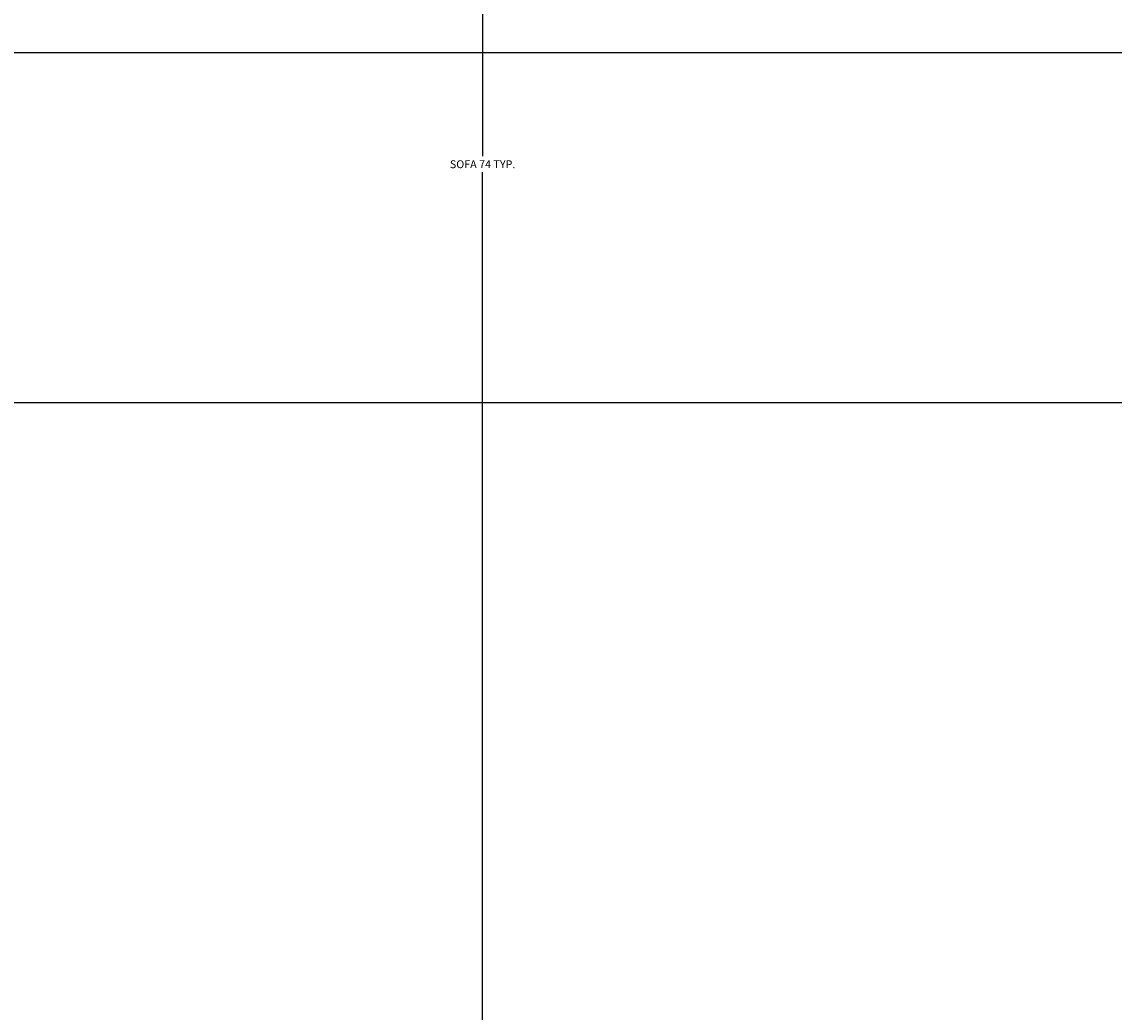
# Model space of a CAD drawing. Units: inches. Extents: x 1998 to 2588, y 1139 to 1977.
# Tile 46 of 134: x 2257 to 2282, y 1615 to 1637. Entities that reach past the tile are written whole.
import ezdxf

# ---------------------------------------------------------------- set-up
doc = ezdxf.new("R2010")
doc.units = ezdxf.units.IN
doc.layers.add('A-ANNO-DIMS', color=2, linetype='Continuous', lineweight=18)
doc.styles.get("Standard").update_dxf_attribs({"font": 'arial.ttf'})
doc.dimstyles.get("Standard").update_dxf_attribs({"dimtxt": 0.18, "dimasz": 0.18, "dimexe": 0.18, "dimexo": 0.0625, "dimgap": 0.09, "dimtad": 0, "dimtih": 1, "dimtoh": 1, "dimdec": 4, "dimzin": 0, "dimdsep": 46, "dimtxsty": 'Standard', "dimcen": 0.09, "dimadec": 0, "dimazin": 0, "dimtfac": 1, "dimtdec": 4, "dimtofl": 0, "dimtmove": 0, "dimatfit": 3, "dimfxl": 1, "dimtolj": 1, "dimtzin": 0, "dimarcsym": 0})

# ---------------------------------------------------------------- blocks, each defined once
blk = doc.blocks.new('*D11')
at = {"layer": 'A-ANNO-DIMS', "color": 0, "lineweight": -2, "transparency": 16777216}
for p, q in [((2256.378, 1671.356), (2267.646, 1671.356)), ((2267.466, 1671.176), (2267.466, 1634.372)), ((2267.466, 1597.201), (2267.466, 1634.005)), ((2256.378, 1597.021), (2267.646, 1597.021))]:
    blk.add_line(p, q, dxfattribs=at)
at = {"layer": 'A-ANNO-DIMS', "color": 0, "transparency": 16777216}
for points in [[(2267.436, 1671.176), (2267.496, 1671.176), (2267.466, 1671.356)], [(2267.436, 1597.201), (2267.496, 1597.201), (2267.466, 1597.021)]]:
    blk.add_solid(points, dxfattribs=at)
at = {"layer": 'Defpoints', "color": 0, "transparency": 16777216}
for p in [(2256.316, 1671.356), (2256.316, 1597.021), (2267.466, 1597.021)]:
    blk.add_point(p, dxfattribs=at)
at = {"layer": 'A-ANNO-DIMS', "color": 0, "transparency": 16777216, "insert": (2267.466, 1634.189), "char_height": 0.18, "attachment_point": 5}
blk.add_mtext('\\A1;SOFA 74 TYP.', dxfattribs=at)
blk = doc.blocks.new('*D30')
at = {"layer": 'A-ANNO-DIMS', "color": 0, "lineweight": -2, "transparency": 16777216}
for p, q in [((2407.91, 1636.732), (1997.843, 1636.732)), ((1998.023, 1636.552), (1998.023, 1615.913)), ((1998.023, 1594.912), (1998.023, 1615.552)), ((2407.91, 1594.732), (1997.843, 1594.732))]:
    blk.add_line(p, q, dxfattribs=at)
at = {"layer": 'A-ANNO-DIMS', "color": 0, "transparency": 16777216}
for points in [[(1997.993, 1636.552), (1998.053, 1636.552), (1998.023, 1636.732)], [(1997.993, 1594.912), (1998.053, 1594.912), (1998.023, 1594.732)]]:
    blk.add_solid(points, dxfattribs=at)
at = {"layer": 'Defpoints', "color": 0, "transparency": 16777216}
for p in [(1998.023, 1636.732), (2407.973, 1636.732), (2407.973, 1594.732)]:
    blk.add_point(p, dxfattribs=at)
at = {"layer": 'A-ANNO-DIMS', "color": 0, "transparency": 16777216, "insert": (1998.023, 1615.732), "char_height": 0.18, "attachment_point": 5}
blk.add_mtext('\\A1;42', dxfattribs=at)
blk = doc.blocks.new('*D39')
at = {"layer": 'A-ANNO-DIMS', "color": 0, "lineweight": -2, "transparency": 16777216}
for p, q in [((2115.035, 1628.742), (2588.309, 1628.742)), ((2588.129, 1628.562), (2588.129, 1612.685)), ((2588.129, 1596.444), (2588.129, 1612.321)), ((2115.035, 1596.264), (2588.309, 1596.264))]:
    blk.add_line(p, q, dxfattribs=at)
at = {"layer": 'A-ANNO-DIMS', "color": 0, "transparency": 16777216}
for points in [[(2588.099, 1628.562), (2588.159, 1628.562), (2588.129, 1628.742)], [(2588.099, 1596.444), (2588.159, 1596.444), (2588.129, 1596.264)]]:
    blk.add_solid(points, dxfattribs=at)
at = {"layer": 'Defpoints', "color": 0, "transparency": 16777216}
for p in [(2114.973, 1628.742), (2588.129, 1628.742), (2114.973, 1596.264)]:
    blk.add_point(p, dxfattribs=at)
at = {"layer": 'A-ANNO-DIMS', "color": 0, "transparency": 16777216, "insert": (2588.129, 1612.503), "char_height": 0.18, "attachment_point": 5}
blk.add_mtext('\\A1;32.48', dxfattribs=at)

msp = doc.modelspace()

# ---------------------------------------------------------------- dimensions: what is measured, and where the dimension line sits
at = {"layer": 'A-ANNO-DIMS'}
dim = msp.add_linear_dim(base=(2267.4662, 1597.0205), p1=(2256.3158, 1671.3565), p2=(2256.3158, 1597.0205), angle=270, text='SOFA <> TYP.', dimstyle='Standard', override={"dimdec": 0, "dimlfac": 1, "dimrnd": 0, "dimzin": 0, "dimdsep": 46, "dimlunit": 2}, dxfattribs=at)
dim.commit()
dim.dimension.update_dxf_attribs({"geometry": '*D11', "text_midpoint": (2267.4662, 1634.1885)})
for base, p1, p2, override, picture, middle in [((1998.0229, 1636.7324), (2407.9729, 1594.7324), (2407.9729, 1636.7324), {"dimdec": 0, "dimlfac": 1, "dimrnd": 0, "dimzin": 0, "dimdsep": 46, "dimlunit": 2}, '*D30', (1998.0229, 1615.7324)), ((2588.1286, 1628.7416), (2114.9729, 1596.2642), (2114.9729, 1628.7416), {"dimdec": 2, "dimlfac": 1, "dimrnd": 0, "dimzin": 0, "dimdsep": 46, "dimlunit": 2}, '*D39', (2588.1286, 1612.5029))]:
    dim = msp.add_linear_dim(base=base, p1=p1, p2=p2, angle=90, dimstyle='Standard', override=override, dxfattribs=at)
    dim.commit()
    dim.dimension.update_dxf_attribs({"geometry": picture, "text_midpoint": middle})

doc.saveas('drawing.dxf')
